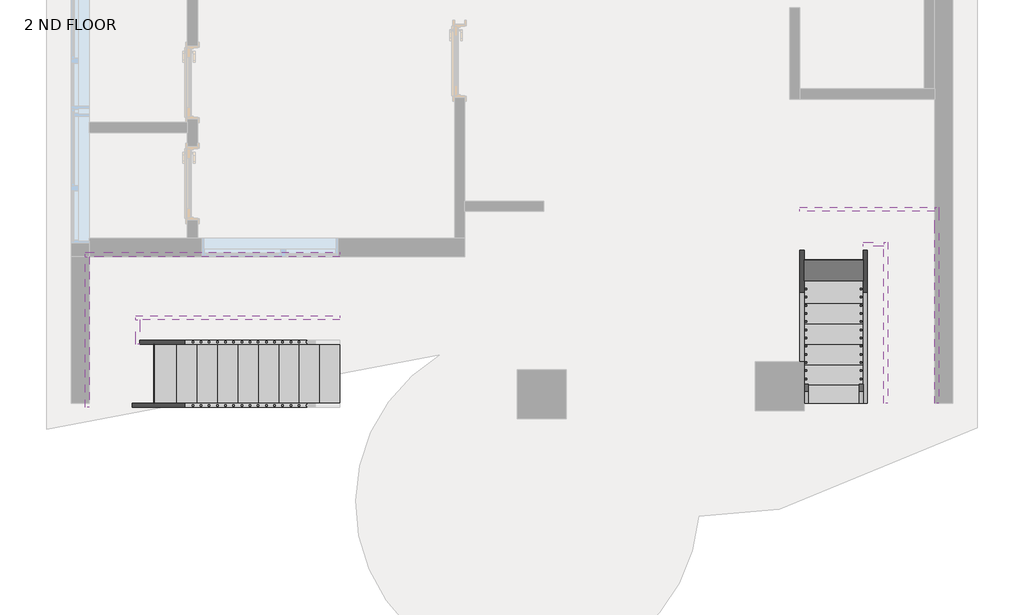
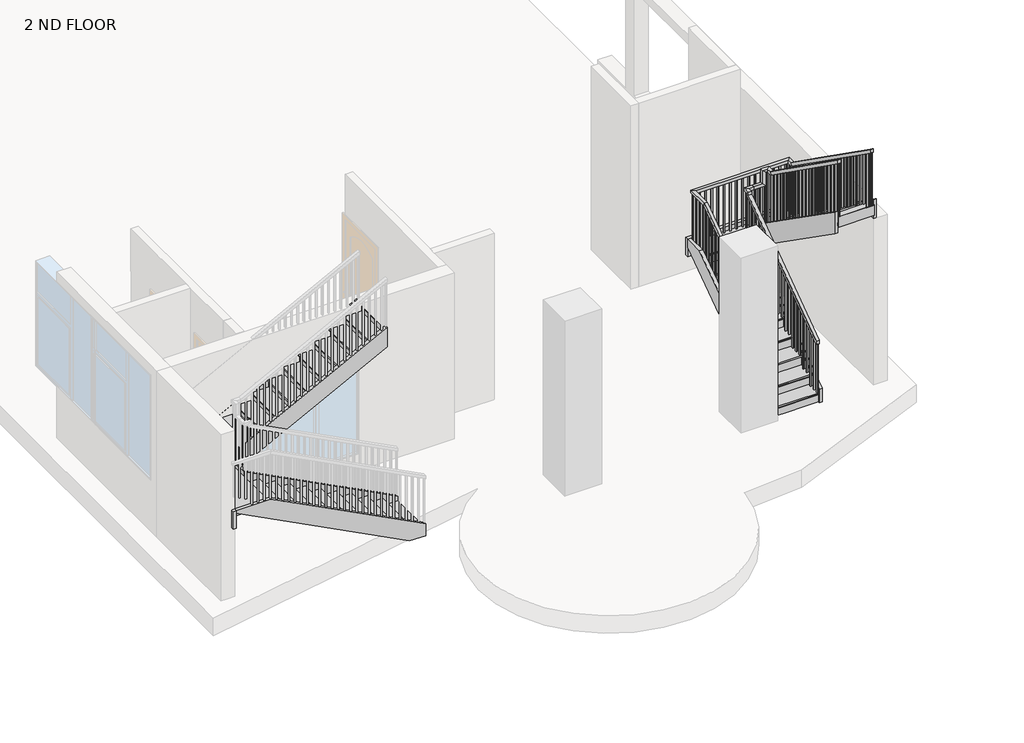
# One storey, part 4 of 4: 12 members, 2 railings, 2 stair flights.
"""IFC4 building model written with IfcOpenShell, lengths in millimetres."""

from ifc_helpers import new_model, si_unit, frame, origin, place, context, project, spatial, polyline, outline, extrude, faceted_brep, transform, mapped, element, save
from components import stair_flight_e10cbaa8, stair_flight_e23070b7

model = new_model("IFC4")

# Units and contexts
model_context = context("Model", 3, world=origin())
ifc_project = project(units=[si_unit("LENGTHUNIT", "METRE", prefix="MILLI")], contexts=[model_context])

# Site, building, storey
site = spatial("IfcSite", under=ifc_project)
building = spatial("IfcBuilding", under=site)
storey = spatial("IfcBuildingStorey", under=building, Name="2 ND FLOOR", Elevation=6400.8)

# Members
placement = place(None, origin())
element("IfcMember", 1, ObjectType="Stringer - 2\" Width", at=placement, inside=storey, context=model_context, shape_type="SweptSolid", body=[
    extrude(outline(polyline([(6400.8, -3117.2664982), (6605.3197081, -3117.2664982), (7924.8, -5663.6319738), (7924.8, -6232.5131972), (7876.2929835, -6232.5131972), (6400.8, -3385.0705974), (6400.8, -3117.2664982)])), frame((0.0, -7701.7822004, 0.0), z_axis=(0.0, 1.0, 0.0), x_axis=(0.0, 0.0, 1.0)), (0.0, 0.0, 1.0), 50.8),
])
element("IfcMember", 2, ObjectType="Stringer - 2\" Width", at=placement, inside=storey, context=model_context, shape_type="SweptSolid", body=[
    extrude(outline(polyline([(-6232.5131972, -7701.7822004), (-6283.3131972, -7701.7822004), (-6283.3131972, -5824.7082131), (-6232.5131972, -5824.7082131), (-6232.5131972, -7701.7822004)])), frame((0.0, 0.0, 7620.0), z_axis=(0.0, 0.0, 1.0), x_axis=(1.0, 0.0, 0.0)), (0.0, 0.0, 1.0), 304.8),
])
element("IfcMember", 3, ObjectType="Stringer - 2\" Width", at=placement, inside=storey, context=model_context, shape_type="SweptSolid", body=[
    extrude(outline(polyline([(7728.7136913, -6283.3131972), (7620.0, -6283.3131972), (7620.0, -5830.6202937), (9026.0106031, -3117.2664982), (9369.3015263, -3117.2664982), (7728.7136913, -6283.3131972)])), frame((0.0, -5824.7082131, 0.0), z_axis=(0.0, 1.0, 0.0), x_axis=(0.0, 0.0, 1.0)), (0.0, 0.0, 1.0), 50.8),
])
element("IfcMember", 4, ObjectType="Stringer - 2\" Width", at=placement, inside=storey, context=model_context, shape_type="SweptSolid", body=[
    extrude(outline(polyline([(6400.8, -3117.2664982), (6605.3197081, -3117.2664982), (7895.1778899, -5606.4664982), (7551.8869668, -5606.4664982), (6400.8, -3385.0705974), (6400.8, -3117.2664982)])), frame((0.0, -6914.3822004, 0.0), z_axis=(0.0, 1.0, 0.0), x_axis=(0.0, 0.0, 1.0)), (0.0, 0.0, 1.0), 50.8),
])
element("IfcMember", 5, ObjectType="Stringer - 2\" Width", at=placement, inside=storey, context=model_context, shape_type="SweptSolid", body=[
    extrude(outline(polyline([(-5606.4664982, -6914.3822004), (-5657.2664982, -6914.3822004), (-5657.2664982, -6609.5822004), (-5606.4664982, -6609.5822004), (-5606.4664982, -6914.3822004)])), frame((0.0, 0.0, 7620.0), z_axis=(0.0, 0.0, 1.0), x_axis=(1.0, 0.0, 0.0)), (0.0, 0.0, 1.0), 304.8),
])
element("IfcMember", 6, ObjectType="Stringer - 2\" Width", at=placement, inside=storey, context=model_context, shape_type="SweptSolid", body=[
    extrude(outline(polyline([(8053.1197081, -5657.2664982), (7709.8287849, -5657.2664982), (9026.0106031, -3117.2664982), (9369.3015263, -3117.2664982), (8053.1197081, -5657.2664982)])), frame((0.0, -6609.5822004, 0.0), z_axis=(0.0, 1.0, 0.0), x_axis=(0.0, 0.0, 1.0)), (0.0, 0.0, 1.0), 50.8),
])
element("IfcMember", 7, ObjectType="Stringer - 2\" Width", at=placement, inside=storey, context=model_context, shape_type="SweptSolid", body=[
    extrude(outline(polyline([(-7650.9822004, 6400.8), (-7650.9822004, 6640.099187), (-5597.981039, 8077.2), (-5263.3822004, 8077.2), (-5263.3822004, 7939.3633718), (-7461.3298744, 6400.8), (-7650.9822004, 6400.8)])), frame((2606.6891134, 0.0, 0.0), z_axis=(1.0, 0.0, 0.0), x_axis=(0.0, 1.0, 0.0)), (0.0, 0.0, 1.0), 50.8),
])
element("IfcMember", 8, ObjectType="Stringer - 2\" Width", at=placement, inside=storey, context=model_context, shape_type="SweptSolid", body=[
    extrude(outline(polyline([(2606.6891134, -5263.3822004), (2606.6891134, -5212.5822004), (4281.7311655, -5212.5822004), (4281.7311655, -5263.3822004), (2606.6891134, -5263.3822004)])), frame((0.0, 0.0, 7772.4), z_axis=(0.0, 0.0, 1.0), x_axis=(1.0, 0.0, 0.0)), (0.0, 0.0, 1.0), 304.8),
])
element("IfcMember", 9, ObjectType="Stringer - 2\" Width", at=placement, inside=storey, context=model_context, shape_type="SweptSolid", body=[
    extrude(outline(polyline([(-5212.5822004, 7920.259187), (-5212.5822004, 7772.4), (-5532.8630978, 7772.4), (-7650.9822004, 9255.0833718), (-7650.9822004, 9627.139187), (-5212.5822004, 7920.259187)])), frame((4281.7311655, 0.0, 0.0), z_axis=(1.0, 0.0, 0.0), x_axis=(0.0, 1.0, 0.0)), (0.0, 0.0, 1.0), 50.8),
])
element("IfcMember", 10, ObjectType="Stringer - 2\" Width", at=placement, inside=storey, context=model_context, shape_type="SweptSolid", body=[
    extrude(outline(polyline([(-7650.9822004, 6400.8), (-7650.9822004, 6640.099187), (-5695.1822004, 8009.159187), (-5695.1822004, 7637.1033718), (-7461.3298744, 6400.8), (-7650.9822004, 6400.8)])), frame((3394.0891134, 0.0, 0.0), z_axis=(1.0, 0.0, 0.0), x_axis=(0.0, 1.0, 0.0)), (0.0, 0.0, 1.0), 50.8),
])
element("IfcMember", 11, ObjectType="Stringer - 2\" Width", at=placement, inside=storey, context=model_context, shape_type="SweptSolid", body=[
    extrude(outline(polyline([(3394.0891134, -5695.1822004), (3394.0891134, -5644.3822004), (3648.0891134, -5644.3822004), (3648.0891134, -5695.1822004), (3394.0891134, -5695.1822004)])), frame((0.0, 0.0, 7772.4), z_axis=(0.0, 0.0, 1.0), x_axis=(1.0, 0.0, 0.0)), (0.0, 0.0, 1.0), 304.8),
])
element("IfcMember", 12, ObjectType="Stringer - 2\" Width", at=placement, inside=storey, context=model_context, shape_type="SweptSolid", body=[
    extrude(outline(polyline([(-5644.3822004, 8222.519187), (-5644.3822004, 7850.4633718), (-7650.9822004, 9255.0833718), (-7650.9822004, 9627.139187), (-5644.3822004, 8222.519187)])), frame((3648.0891134, 0.0, 0.0), z_axis=(1.0, 0.0, 0.0), x_axis=(0.0, 1.0, 0.0)), (0.0, 0.0, 1.0), 50.8),
])

# Railings
element("IfcRailing", 13, ObjectType="Handrail - Rectangular", at=placement, inside=storey, context=model_context, shape_type="SolidModel", body=[
    faceted_brep([(3343.2891134, -7650.9822004, 7493.0), (3343.2891134, -7650.9822004, 7430.7314749), (3394.0891134, -7650.9822004, 7430.7314749), (3394.0891134, -7650.9822004, 7493.0), (3343.2891134, -5720.5822004, 8861.3848101), (3343.2891134, -5669.7822004, 8835.1264116), (3394.0891134, -5669.7822004, 8835.1264116), (3394.0891134, -5720.5822004, 8861.3848101), (3343.2891134, -5720.5822004, 8915.4), (3343.2891134, -5669.7822004, 8864.6), (3394.0891134, -5669.7822004, 8864.6), (3394.0891134, -5720.5822004, 8915.4), (3343.2891134, -5593.5822004, 8915.4), (3343.2891134, -5593.5822004, 8864.6), (3394.0891134, -5644.3822004, 8864.6), (3394.0891134, -5644.3822004, 8915.4), (3470.2891134, -5593.5822004, 8915.4), (3470.2891134, -5593.5822004, 8864.6), (3470.2891134, -5644.3822004, 8864.6), (3470.2891134, -5644.3822004, 8915.4), (3622.6891134, -5593.5822004, 8915.4), (3673.4891134, -5593.5822004, 8864.6), (3673.4891134, -5644.3822004, 8864.6), (3622.6891134, -5644.3822004, 8915.4), (3622.6891134, -5593.5822004, 9147.2151899), (3673.4891134, -5593.5822004, 9096.4151899), (3673.4891134, -5644.3822004, 9096.4151899), (3622.6891134, -5644.3822004, 9147.2151899), (3749.6891134, -5593.5822004, 9147.2151899), (3749.6891134, -5593.5822004, 9096.4151899), (3698.8891134, -5644.3822004, 9096.4151899), (3698.8891134, -5644.3822004, 9147.2151899), (3749.6891134, -5720.5822004, 9147.2151899), (3749.6891134, -5736.7610126, 9096.4151899), (3698.8891134, -5736.7610126, 9096.4151899), (3698.8891134, -5720.5822004, 9147.2151899), (3749.6891134, -7650.9822004, 10515.6), (3698.8891134, -7650.9822004, 10515.6), (3698.8891134, -7650.9822004, 10453.3314749), (3749.6891134, -7650.9822004, 10453.3314749)], [[[0, 1, 2, 3]], [[1, 0, 4, 5]], [[2, 1, 5, 6]], [[3, 2, 6, 7]], [[0, 3, 7, 4]], [[5, 4, 8, 9]], [[6, 5, 9, 10]], [[7, 6, 10, 11]], [[4, 7, 11, 8]], [[9, 8, 12, 13]], [[10, 9, 13, 14]], [[11, 10, 14, 15]], [[8, 11, 15, 12]], [[13, 12, 16, 17]], [[14, 13, 17, 18]], [[15, 14, 18, 19]], [[12, 15, 19, 16]], [[17, 16, 20, 21]], [[18, 17, 21, 22]], [[19, 18, 22, 23]], [[16, 19, 23, 20]], [[21, 20, 24, 25]], [[22, 21, 25, 26]], [[23, 22, 26, 27]], [[20, 23, 27, 24]], [[25, 24, 28, 29]], [[26, 25, 29, 30]], [[27, 26, 30, 31]], [[24, 27, 31, 28]], [[29, 28, 32, 33]], [[30, 29, 33, 34]], [[31, 30, 34, 35]], [[28, 31, 35, 32]], [[36, 37, 38, 39]], [[33, 32, 36, 39]], [[34, 33, 39, 38]], [[35, 34, 38, 37]], [[32, 35, 37, 36]]]),
    extrude(outline(polyline([(-7558.9072004, 10388.0631205), (-7539.8572004, 10374.559323), (-7539.8572004, 9423.4), (-7558.9072004, 9423.4), (-7558.9072004, 10388.0631205)])), frame((3714.7641134, 0.0, 0.0), z_axis=(1.0, 0.0, 0.0), x_axis=(0.0, 1.0, 0.0)), (0.0, 0.0, 1.0), 19.05),
    extrude(outline(polyline([(-7457.3072004, 10316.0428673), (-7438.2572004, 10302.5390699), (-7438.2572004, 9423.4), (-7457.3072004, 9423.4), (-7457.3072004, 10316.0428673)])), frame((3714.7641134, 0.0, 0.0), z_axis=(1.0, 0.0, 0.0), x_axis=(0.0, 1.0, 0.0)), (0.0, 0.0, 1.0), 19.05),
    extrude(outline(polyline([(-7355.7072004, 10244.0226142), (-7336.6572004, 10230.5188167), (-7336.6572004, 9245.6), (-7355.7072004, 9245.6), (-7355.7072004, 10244.0226142)])), frame((3714.7641134, 0.0, 0.0), z_axis=(1.0, 0.0, 0.0), x_axis=(0.0, 1.0, 0.0)), (0.0, 0.0, 1.0), 19.05),
    extrude(outline(polyline([(-7254.1072004, 10172.002361), (-7235.0572004, 10158.4985635), (-7235.0572004, 9245.6), (-7254.1072004, 9245.6), (-7254.1072004, 10172.002361)])), frame((3714.7641134, 0.0, 0.0), z_axis=(1.0, 0.0, 0.0), x_axis=(0.0, 1.0, 0.0)), (0.0, 0.0, 1.0), 19.05),
    extrude(outline(polyline([(-7152.5072004, 10099.9821078), (-7133.4572004, 10086.4783104), (-7133.4572004, 9067.8), (-7152.5072004, 9067.8), (-7152.5072004, 10099.9821078)])), frame((3714.7641134, 0.0, 0.0), z_axis=(1.0, 0.0, 0.0), x_axis=(0.0, 1.0, 0.0)), (0.0, 0.0, 1.0), 19.05),
    extrude(outline(polyline([(-7050.9072004, 10027.9618547), (-7031.8572004, 10014.4580572), (-7031.8572004, 9067.8), (-7050.9072004, 9067.8), (-7050.9072004, 10027.9618547)])), frame((3714.7641134, 0.0, 0.0), z_axis=(1.0, 0.0, 0.0), x_axis=(0.0, 1.0, 0.0)), (0.0, 0.0, 1.0), 19.05),
    extrude(outline(polyline([(-6949.3072004, 9955.9416015), (-6930.2572004, 9942.437804), (-6930.2572004, 9067.8), (-6949.3072004, 9067.8), (-6949.3072004, 9955.9416015)])), frame((3714.7641134, 0.0, 0.0), z_axis=(1.0, 0.0, 0.0), x_axis=(0.0, 1.0, 0.0)), (0.0, 0.0, 1.0), 19.05),
    extrude(outline(polyline([(-6847.7072004, 9883.9213483), (-6828.6572004, 9870.4175509), (-6828.6572004, 8890.0), (-6847.7072004, 8890.0), (-6847.7072004, 9883.9213483)])), frame((3714.7641134, 0.0, 0.0), z_axis=(1.0, 0.0, 0.0), x_axis=(0.0, 1.0, 0.0)), (0.0, 0.0, 1.0), 19.05),
    extrude(outline(polyline([(-6746.1072004, 9811.9010952), (-6727.0572004, 9798.3972977), (-6727.0572004, 8890.0), (-6746.1072004, 8890.0), (-6746.1072004, 9811.9010952)])), frame((3714.7641134, 0.0, 0.0), z_axis=(1.0, 0.0, 0.0), x_axis=(0.0, 1.0, 0.0)), (0.0, 0.0, 1.0), 19.05),
    extrude(outline(polyline([(-6644.5072004, 9739.880842), (-6625.4572004, 9726.3770445), (-6625.4572004, 8712.2), (-6644.5072004, 8712.2), (-6644.5072004, 9739.880842)])), frame((3714.7641134, 0.0, 0.0), z_axis=(1.0, 0.0, 0.0), x_axis=(0.0, 1.0, 0.0)), (0.0, 0.0, 1.0), 19.05),
    extrude(outline(polyline([(-6542.9072004, 9667.8605888), (-6523.8572004, 9654.3567914), (-6523.8572004, 8712.2), (-6542.9072004, 8712.2), (-6542.9072004, 9667.8605888)])), frame((3714.7641134, 0.0, 0.0), z_axis=(1.0, 0.0, 0.0), x_axis=(0.0, 1.0, 0.0)), (0.0, 0.0, 1.0), 19.05),
    extrude(outline(polyline([(-6441.3072004, 9595.8403357), (-6422.2572004, 9582.3365382), (-6422.2572004, 8712.2), (-6441.3072004, 8712.2), (-6441.3072004, 9595.8403357)])), frame((3714.7641134, 0.0, 0.0), z_axis=(1.0, 0.0, 0.0), x_axis=(0.0, 1.0, 0.0)), (0.0, 0.0, 1.0), 19.05),
    extrude(outline(polyline([(-6339.7072004, 9523.8200825), (-6320.6572004, 9510.316285), (-6320.6572004, 8534.4), (-6339.7072004, 8534.4), (-6339.7072004, 9523.8200825)])), frame((3714.7641134, 0.0, 0.0), z_axis=(1.0, 0.0, 0.0), x_axis=(0.0, 1.0, 0.0)), (0.0, 0.0, 1.0), 19.05),
    extrude(outline(polyline([(-6238.1072004, 9451.7998293), (-6219.0572004, 9438.2960319), (-6219.0572004, 8534.4), (-6238.1072004, 8534.4), (-6238.1072004, 9451.7998293)])), frame((3714.7641134, 0.0, 0.0), z_axis=(1.0, 0.0, 0.0), x_axis=(0.0, 1.0, 0.0)), (0.0, 0.0, 1.0), 19.05),
    extrude(outline(polyline([(-6136.5072004, 9379.7795762), (-6117.4572004, 9366.2757787), (-6117.4572004, 8356.6), (-6136.5072004, 8356.6), (-6136.5072004, 9379.7795762)])), frame((3714.7641134, 0.0, 0.0), z_axis=(1.0, 0.0, 0.0), x_axis=(0.0, 1.0, 0.0)), (0.0, 0.0, 1.0), 19.05),
    extrude(outline(polyline([(-6034.9072004, 9307.759323), (-6015.8572004, 9294.2555255), (-6015.8572004, 8356.6), (-6034.9072004, 8356.6), (-6034.9072004, 9307.759323)])), frame((3714.7641134, 0.0, 0.0), z_axis=(1.0, 0.0, 0.0), x_axis=(0.0, 1.0, 0.0)), (0.0, 0.0, 1.0), 19.05),
    extrude(outline(polyline([(-5933.3072004, 9235.7390699), (-5914.2572004, 9222.2352724), (-5914.2572004, 8356.6), (-5933.3072004, 8356.6), (-5933.3072004, 9235.7390699)])), frame((3714.7641134, 0.0, 0.0), z_axis=(1.0, 0.0, 0.0), x_axis=(0.0, 1.0, 0.0)), (0.0, 0.0, 1.0), 19.05),
    extrude(outline(polyline([(-5831.7072004, 9163.7188167), (-5812.6572004, 9150.2150192), (-5812.6572004, 8178.8), (-5831.7072004, 8178.8), (-5831.7072004, 9163.7188167)])), frame((3714.7641134, 0.0, 0.0), z_axis=(1.0, 0.0, 0.0), x_axis=(0.0, 1.0, 0.0)), (0.0, 0.0, 1.0), 19.05),
    extrude(outline(polyline([(-5730.1072004, 9091.6985635), (-5711.0572004, 9078.1947661), (-5711.0572004, 8178.8), (-5730.1072004, 8178.8), (-5730.1072004, 9091.6985635)])), frame((3714.7641134, 0.0, 0.0), z_axis=(1.0, 0.0, 0.0), x_axis=(0.0, 1.0, 0.0)), (0.0, 0.0, 1.0), 19.05),
    extrude(outline(polyline([(3663.9641134, -5628.5072004), (3663.9641134, -5609.4572004), (3683.0141134, -5609.4572004), (3683.0141134, -5628.5072004), (3663.9641134, -5628.5072004)])), frame((0.0, 0.0, 8001.0), z_axis=(0.0, 0.0, 1.0), x_axis=(1.0, 0.0, 0.0)), (0.0, 0.0, 1.0), 1095.4151899),
    extrude(outline(polyline([(3562.3641134, -5628.5072004), (3562.3641134, -5609.4572004), (3581.4141134, -5609.4572004), (3581.4141134, -5628.5072004), (3562.3641134, -5628.5072004)])), frame((0.0, 0.0, 8001.0), z_axis=(0.0, 0.0, 1.0), x_axis=(1.0, 0.0, 0.0)), (0.0, 0.0, 1.0), 863.6),
    extrude(outline(polyline([(3460.7641134, -5628.5072004), (3460.7641134, -5609.4572004), (3479.8141134, -5609.4572004), (3479.8141134, -5628.5072004), (3460.7641134, -5628.5072004)])), frame((0.0, 0.0, 8001.0), z_axis=(0.0, 0.0, 1.0), x_axis=(1.0, 0.0, 0.0)), (0.0, 0.0, 1.0), 863.6),
    extrude(outline(polyline([(-5730.1072004, 8792.3643863), (-5711.0572004, 8805.8681838), (-5711.0572004, 7823.2), (-5730.1072004, 7823.2), (-5730.1072004, 8792.3643863)])), frame((3359.1641134, 0.0, 0.0), z_axis=(1.0, 0.0, 0.0), x_axis=(0.0, 1.0, 0.0)), (0.0, 0.0, 1.0), 19.05),
    extrude(outline(polyline([(-5831.7072004, 8720.3441331), (-5812.6572004, 8733.8479306), (-5812.6572004, 7823.2), (-5831.7072004, 7823.2), (-5831.7072004, 8720.3441331)])), frame((3359.1641134, 0.0, 0.0), z_axis=(1.0, 0.0, 0.0), x_axis=(0.0, 1.0, 0.0)), (0.0, 0.0, 1.0), 19.05),
    extrude(outline(polyline([(-5933.3072004, 8648.32388), (-5914.2572004, 8661.8276774), (-5914.2572004, 7645.4), (-5933.3072004, 7645.4), (-5933.3072004, 8648.32388)])), frame((3359.1641134, 0.0, 0.0), z_axis=(1.0, 0.0, 0.0), x_axis=(0.0, 1.0, 0.0)), (0.0, 0.0, 1.0), 19.05),
    extrude(outline(polyline([(-6034.9072004, 8576.3036268), (-6015.8572004, 8589.8074243), (-6015.8572004, 7645.4), (-6034.9072004, 7645.4), (-6034.9072004, 8576.3036268)])), frame((3359.1641134, 0.0, 0.0), z_axis=(1.0, 0.0, 0.0), x_axis=(0.0, 1.0, 0.0)), (0.0, 0.0, 1.0), 19.05),
    extrude(outline(polyline([(-6136.5072004, 8504.2833736), (-6117.4572004, 8517.7871711), (-6117.4572004, 7645.4), (-6136.5072004, 7645.4), (-6136.5072004, 8504.2833736)])), frame((3359.1641134, 0.0, 0.0), z_axis=(1.0, 0.0, 0.0), x_axis=(0.0, 1.0, 0.0)), (0.0, 0.0, 1.0), 19.05),
    extrude(outline(polyline([(-6238.1072004, 8432.2631205), (-6219.0572004, 8445.766918), (-6219.0572004, 7467.6), (-6238.1072004, 7467.6), (-6238.1072004, 8432.2631205)])), frame((3359.1641134, 0.0, 0.0), z_axis=(1.0, 0.0, 0.0), x_axis=(0.0, 1.0, 0.0)), (0.0, 0.0, 1.0), 19.05),
    extrude(outline(polyline([(-6339.7072004, 8360.2428673), (-6320.6572004, 8373.7466648), (-6320.6572004, 7467.6), (-6339.7072004, 7467.6), (-6339.7072004, 8360.2428673)])), frame((3359.1641134, 0.0, 0.0), z_axis=(1.0, 0.0, 0.0), x_axis=(0.0, 1.0, 0.0)), (0.0, 0.0, 1.0), 19.05),
    extrude(outline(polyline([(-6441.3072004, 8288.2226142), (-6422.2572004, 8301.7264116), (-6422.2572004, 7289.8), (-6441.3072004, 7289.8), (-6441.3072004, 8288.2226142)])), frame((3359.1641134, 0.0, 0.0), z_axis=(1.0, 0.0, 0.0), x_axis=(0.0, 1.0, 0.0)), (0.0, 0.0, 1.0), 19.05),
    extrude(outline(polyline([(-6542.9072004, 8216.202361), (-6523.8572004, 8229.7061585), (-6523.8572004, 7289.8), (-6542.9072004, 7289.8), (-6542.9072004, 8216.202361)])), frame((3359.1641134, 0.0, 0.0), z_axis=(1.0, 0.0, 0.0), x_axis=(0.0, 1.0, 0.0)), (0.0, 0.0, 1.0), 19.05),
    extrude(outline(polyline([(-6644.5072004, 8144.1821078), (-6625.4572004, 8157.6859053), (-6625.4572004, 7289.8), (-6644.5072004, 7289.8), (-6644.5072004, 8144.1821078)])), frame((3359.1641134, 0.0, 0.0), z_axis=(1.0, 0.0, 0.0), x_axis=(0.0, 1.0, 0.0)), (0.0, 0.0, 1.0), 19.05),
    extrude(outline(polyline([(-6746.1072004, 8072.1618547), (-6727.0572004, 8085.6656521), (-6727.0572004, 7112.0), (-6746.1072004, 7112.0), (-6746.1072004, 8072.1618547)])), frame((3359.1641134, 0.0, 0.0), z_axis=(1.0, 0.0, 0.0), x_axis=(0.0, 1.0, 0.0)), (0.0, 0.0, 1.0), 19.05),
    extrude(outline(polyline([(-6847.7072004, 8000.1416015), (-6828.6572004, 8013.645399), (-6828.6572004, 7112.0), (-6847.7072004, 7112.0), (-6847.7072004, 8000.1416015)])), frame((3359.1641134, 0.0, 0.0), z_axis=(1.0, 0.0, 0.0), x_axis=(0.0, 1.0, 0.0)), (0.0, 0.0, 1.0), 19.05),
    extrude(outline(polyline([(-6949.3072004, 7928.1213483), (-6930.2572004, 7941.6251458), (-6930.2572004, 6934.2), (-6949.3072004, 6934.2), (-6949.3072004, 7928.1213483)])), frame((3359.1641134, 0.0, 0.0), z_axis=(1.0, 0.0, 0.0), x_axis=(0.0, 1.0, 0.0)), (0.0, 0.0, 1.0), 19.05),
    extrude(outline(polyline([(-7050.9072004, 7856.1010952), (-7031.8572004, 7869.6048926), (-7031.8572004, 6934.2), (-7050.9072004, 6934.2), (-7050.9072004, 7856.1010952)])), frame((3359.1641134, 0.0, 0.0), z_axis=(1.0, 0.0, 0.0), x_axis=(0.0, 1.0, 0.0)), (0.0, 0.0, 1.0), 19.05),
    extrude(outline(polyline([(-7152.5072004, 7784.080842), (-7133.4572004, 7797.5846395), (-7133.4572004, 6934.2), (-7152.5072004, 6934.2), (-7152.5072004, 7784.080842)])), frame((3359.1641134, 0.0, 0.0), z_axis=(1.0, 0.0, 0.0), x_axis=(0.0, 1.0, 0.0)), (0.0, 0.0, 1.0), 19.05),
    extrude(outline(polyline([(-7254.1072004, 7712.0605888), (-7235.0572004, 7725.5643863), (-7235.0572004, 6756.4), (-7254.1072004, 6756.4), (-7254.1072004, 7712.0605888)])), frame((3359.1641134, 0.0, 0.0), z_axis=(1.0, 0.0, 0.0), x_axis=(0.0, 1.0, 0.0)), (0.0, 0.0, 1.0), 19.05),
    extrude(outline(polyline([(-7355.7072004, 7640.0403357), (-7336.6572004, 7653.5441331), (-7336.6572004, 6756.4), (-7355.7072004, 6756.4), (-7355.7072004, 7640.0403357)])), frame((3359.1641134, 0.0, 0.0), z_axis=(1.0, 0.0, 0.0), x_axis=(0.0, 1.0, 0.0)), (0.0, 0.0, 1.0), 19.05),
    extrude(outline(polyline([(-7457.3072004, 7568.0200825), (-7438.2572004, 7581.52388), (-7438.2572004, 6578.6), (-7457.3072004, 6578.6), (-7457.3072004, 7568.0200825)])), frame((3359.1641134, 0.0, 0.0), z_axis=(1.0, 0.0, 0.0), x_axis=(0.0, 1.0, 0.0)), (0.0, 0.0, 1.0), 19.05),
    extrude(outline(polyline([(-7558.9072004, 7495.9998293), (-7539.8572004, 7509.5036268), (-7539.8572004, 6578.6), (-7558.9072004, 6578.6), (-7558.9072004, 7495.9998293)])), frame((3359.1641134, 0.0, 0.0), z_axis=(1.0, 0.0, 0.0), x_axis=(0.0, 1.0, 0.0)), (0.0, 0.0, 1.0), 19.05),
    extrude(outline(polyline([(3714.7641134, -5628.5072004), (3714.7641134, -5609.4572004), (3733.8141134, -5609.4572004), (3733.8141134, -5628.5072004), (3714.7641134, -5628.5072004)])), frame((0.0, 0.0, 8001.0), z_axis=(0.0, 0.0, 1.0), x_axis=(1.0, 0.0, 0.0)), (0.0, 0.0, 1.0), 1095.4151899),
    extrude(outline(polyline([(3378.2141134, -5628.5072004), (3359.1641134, -5628.5072004), (3359.1641134, -5609.4572004), (3378.2141134, -5609.4572004), (3378.2141134, -5628.5072004)])), frame((0.0, 0.0, 8001.0), z_axis=(0.0, 0.0, 1.0), x_axis=(1.0, 0.0, 0.0)), (0.0, 0.0, 1.0), 863.6),
    extrude(outline(polyline([(-7650.9822004, 10453.3314749), (-7631.9322004, 10439.8276774), (-7631.9322004, 9423.4), (-7650.9822004, 9423.4), (-7650.9822004, 10453.3314749)])), frame((3714.7641134, 0.0, 0.0), z_axis=(1.0, 0.0, 0.0), x_axis=(0.0, 1.0, 0.0)), (0.0, 0.0, 1.0), 19.05),
    extrude(outline(polyline([(-7650.9822004, 7430.7314749), (-7631.9322004, 7444.2352724), (-7631.9322004, 6578.6), (-7650.9822004, 6578.6), (-7650.9822004, 7430.7314749)])), frame((3359.1641134, 0.0, 0.0), z_axis=(1.0, 0.0, 0.0), x_axis=(0.0, 1.0, 0.0)), (0.0, 0.0, 1.0), 19.05),
])
element("IfcRailing", 14, ObjectType="Handrail - Rectangular", at=placement, inside=storey, context=model_context, shape_type="SolidModel", body=[
    faceted_brep([(2657.4891134, -7650.9822004, 7493.0), (2657.4891134, -7650.9822004, 7430.7314749), (2708.2891134, -7650.9822004, 7430.7314749), (2708.2891134, -7650.9822004, 7493.0), (2657.4891134, -5644.3822004, 8915.4), (2657.4891134, -5628.2033882, 8864.6), (2708.2891134, -5628.2033882, 8864.6), (2708.2891134, -5644.3822004, 8915.4), (2657.4891134, -5263.3822004, 8915.4), (2657.4891134, -5263.3822004, 8864.6), (2708.2891134, -5314.1822004, 8864.6), (2708.2891134, -5314.1822004, 8915.4), (4281.7311655, -5263.3822004, 8915.4), (4281.7311655, -5263.3822004, 8864.6), (4230.9311655, -5314.1822004, 8864.6), (4230.9311655, -5314.1822004, 8915.4), (4281.7311655, -5393.5572004, 8915.4), (4281.7311655, -5409.7360126, 8864.6), (4230.9311655, -5409.7360126, 8864.6), (4230.9311655, -5393.5572004, 8915.4), (4281.7311655, -7650.9822004, 10515.6), (4230.9311655, -7650.9822004, 10515.6), (4230.9311655, -7650.9822004, 10453.3314749), (4281.7311655, -7650.9822004, 10453.3314749)], [[[0, 1, 2, 3]], [[1, 0, 4, 5]], [[2, 1, 5, 6]], [[3, 2, 6, 7]], [[0, 3, 7, 4]], [[5, 4, 8, 9]], [[6, 5, 9, 10]], [[7, 6, 10, 11]], [[4, 7, 11, 8]], [[9, 8, 12, 13]], [[10, 9, 13, 14]], [[11, 10, 14, 15]], [[8, 11, 15, 12]], [[13, 12, 16, 17]], [[14, 13, 17, 18]], [[15, 14, 18, 19]], [[12, 15, 19, 16]], [[20, 21, 22, 23]], [[17, 16, 20, 23]], [[18, 17, 23, 22]], [[19, 18, 22, 21]], [[16, 19, 21, 20]]]),
    extrude(outline(polyline([(-7616.0572004, 10428.5745129), (-7616.0572004, 9423.4), (-7635.1072004, 9423.4), (-7635.1072004, 10442.0783104), (-7616.0572004, 10428.5745129)])), frame((4246.8061655, 0.0, 0.0), z_axis=(1.0, 0.0, 0.0), x_axis=(0.0, 1.0, 0.0)), (0.0, 0.0, 1.0), 19.05),
    extrude(outline(polyline([(-7514.4572004, 10356.5542597), (-7514.4572004, 9423.4), (-7533.5072004, 9423.4), (-7533.5072004, 10370.0580572), (-7514.4572004, 10356.5542597)])), frame((4246.8061655, 0.0, 0.0), z_axis=(1.0, 0.0, 0.0), x_axis=(0.0, 1.0, 0.0)), (0.0, 0.0, 1.0), 19.05),
    extrude(outline(polyline([(-7412.8572004, 10284.5340066), (-7412.8572004, 9423.4), (-7431.9072004, 9423.4), (-7431.9072004, 10298.037804), (-7412.8572004, 10284.5340066)])), frame((4246.8061655, 0.0, 0.0), z_axis=(1.0, 0.0, 0.0), x_axis=(0.0, 1.0, 0.0)), (0.0, 0.0, 1.0), 19.05),
    extrude(outline(polyline([(-7311.2572004, 10212.5137534), (-7311.2572004, 9245.6), (-7330.3072004, 9245.6), (-7330.3072004, 10226.0175509), (-7311.2572004, 10212.5137534)])), frame((4246.8061655, 0.0, 0.0), z_axis=(1.0, 0.0, 0.0), x_axis=(0.0, 1.0, 0.0)), (0.0, 0.0, 1.0), 19.05),
    extrude(outline(polyline([(-7209.6572004, 10140.4935002), (-7209.6572004, 9245.6), (-7228.7072004, 9245.6), (-7228.7072004, 10153.9972977), (-7209.6572004, 10140.4935002)])), frame((4246.8061655, 0.0, 0.0), z_axis=(1.0, 0.0, 0.0), x_axis=(0.0, 1.0, 0.0)), (0.0, 0.0, 1.0), 19.05),
    extrude(outline(polyline([(-7108.0572004, 10068.4732471), (-7108.0572004, 9067.8), (-7127.1072004, 9067.8), (-7127.1072004, 10081.9770445), (-7108.0572004, 10068.4732471)])), frame((4246.8061655, 0.0, 0.0), z_axis=(1.0, 0.0, 0.0), x_axis=(0.0, 1.0, 0.0)), (0.0, 0.0, 1.0), 19.05),
    extrude(outline(polyline([(-7006.4572004, 9996.4529939), (-7006.4572004, 9067.8), (-7025.5072004, 9067.8), (-7025.5072004, 10009.9567914), (-7006.4572004, 9996.4529939)])), frame((4246.8061655, 0.0, 0.0), z_axis=(1.0, 0.0, 0.0), x_axis=(0.0, 1.0, 0.0)), (0.0, 0.0, 1.0), 19.05),
    extrude(outline(polyline([(-6904.8572004, 9924.4327407), (-6904.8572004, 9067.8), (-6923.9072004, 9067.8), (-6923.9072004, 9937.9365382), (-6904.8572004, 9924.4327407)])), frame((4246.8061655, 0.0, 0.0), z_axis=(1.0, 0.0, 0.0), x_axis=(0.0, 1.0, 0.0)), (0.0, 0.0, 1.0), 19.05),
    extrude(outline(polyline([(-6803.2572004, 9852.4124876), (-6803.2572004, 8890.0), (-6822.3072004, 8890.0), (-6822.3072004, 9865.916285), (-6803.2572004, 9852.4124876)])), frame((4246.8061655, 0.0, 0.0), z_axis=(1.0, 0.0, 0.0), x_axis=(0.0, 1.0, 0.0)), (0.0, 0.0, 1.0), 19.05),
    extrude(outline(polyline([(-6701.6572004, 9780.3922344), (-6701.6572004, 8890.0), (-6720.7072004, 8890.0), (-6720.7072004, 9793.8960319), (-6701.6572004, 9780.3922344)])), frame((4246.8061655, 0.0, 0.0), z_axis=(1.0, 0.0, 0.0), x_axis=(0.0, 1.0, 0.0)), (0.0, 0.0, 1.0), 19.05),
    extrude(outline(polyline([(-6600.0572004, 9708.3719812), (-6600.0572004, 8712.2), (-6619.1072004, 8712.2), (-6619.1072004, 9721.8757787), (-6600.0572004, 9708.3719812)])), frame((4246.8061655, 0.0, 0.0), z_axis=(1.0, 0.0, 0.0), x_axis=(0.0, 1.0, 0.0)), (0.0, 0.0, 1.0), 19.05),
    extrude(outline(polyline([(-6498.4572004, 9636.3517281), (-6498.4572004, 8712.2), (-6517.5072004, 8712.2), (-6517.5072004, 9649.8555255), (-6498.4572004, 9636.3517281)])), frame((4246.8061655, 0.0, 0.0), z_axis=(1.0, 0.0, 0.0), x_axis=(0.0, 1.0, 0.0)), (0.0, 0.0, 1.0), 19.05),
    extrude(outline(polyline([(-6396.8572004, 9564.3314749), (-6396.8572004, 8712.2), (-6415.9072004, 8712.2), (-6415.9072004, 9577.8352724), (-6396.8572004, 9564.3314749)])), frame((4246.8061655, 0.0, 0.0), z_axis=(1.0, 0.0, 0.0), x_axis=(0.0, 1.0, 0.0)), (0.0, 0.0, 1.0), 19.05),
    extrude(outline(polyline([(-6295.2572004, 9492.3112217), (-6295.2572004, 8534.4), (-6314.3072004, 8534.4), (-6314.3072004, 9505.8150192), (-6295.2572004, 9492.3112217)])), frame((4246.8061655, 0.0, 0.0), z_axis=(1.0, 0.0, 0.0), x_axis=(0.0, 1.0, 0.0)), (0.0, 0.0, 1.0), 19.05),
    extrude(outline(polyline([(-6193.6572004, 9420.2909686), (-6193.6572004, 8534.4), (-6212.7072004, 8534.4), (-6212.7072004, 9433.7947661), (-6193.6572004, 9420.2909686)])), frame((4246.8061655, 0.0, 0.0), z_axis=(1.0, 0.0, 0.0), x_axis=(0.0, 1.0, 0.0)), (0.0, 0.0, 1.0), 19.05),
    extrude(outline(polyline([(-6092.0572004, 9348.2707154), (-6092.0572004, 8356.6), (-6111.1072004, 8356.6), (-6111.1072004, 9361.7745129), (-6092.0572004, 9348.2707154)])), frame((4246.8061655, 0.0, 0.0), z_axis=(1.0, 0.0, 0.0), x_axis=(0.0, 1.0, 0.0)), (0.0, 0.0, 1.0), 19.05),
    extrude(outline(polyline([(-5990.4572004, 9276.2504623), (-5990.4572004, 8356.6), (-6009.5072004, 8356.6), (-6009.5072004, 9289.7542597), (-5990.4572004, 9276.2504623)])), frame((4246.8061655, 0.0, 0.0), z_axis=(1.0, 0.0, 0.0), x_axis=(0.0, 1.0, 0.0)), (0.0, 0.0, 1.0), 19.05),
    extrude(outline(polyline([(-5888.8572004, 9204.2302091), (-5888.8572004, 8356.6), (-5907.9072004, 8356.6), (-5907.9072004, 9217.7340066), (-5888.8572004, 9204.2302091)])), frame((4246.8061655, 0.0, 0.0), z_axis=(1.0, 0.0, 0.0), x_axis=(0.0, 1.0, 0.0)), (0.0, 0.0, 1.0), 19.05),
    extrude(outline(polyline([(-5787.2572004, 9132.2099559), (-5787.2572004, 8178.8), (-5806.3072004, 8178.8), (-5806.3072004, 9145.7137534), (-5787.2572004, 9132.2099559)])), frame((4246.8061655, 0.0, 0.0), z_axis=(1.0, 0.0, 0.0), x_axis=(0.0, 1.0, 0.0)), (0.0, 0.0, 1.0), 19.05),
    extrude(outline(polyline([(-5685.6572004, 9060.1897028), (-5685.6572004, 8178.8), (-5704.7072004, 8178.8), (-5704.7072004, 9073.6935002), (-5685.6572004, 9060.1897028)])), frame((4246.8061655, 0.0, 0.0), z_axis=(1.0, 0.0, 0.0), x_axis=(0.0, 1.0, 0.0)), (0.0, 0.0, 1.0), 19.05),
    extrude(outline(polyline([(-5584.0572004, 8988.1694496), (-5584.0572004, 8001.0), (-5603.1072004, 8001.0), (-5603.1072004, 9001.6732471), (-5584.0572004, 8988.1694496)])), frame((4246.8061655, 0.0, 0.0), z_axis=(1.0, 0.0, 0.0), x_axis=(0.0, 1.0, 0.0)), (0.0, 0.0, 1.0), 19.05),
    extrude(outline(polyline([(-5482.4572004, 8916.1491964), (-5482.4572004, 8001.0), (-5501.5072004, 8001.0), (-5501.5072004, 8929.6529939), (-5482.4572004, 8916.1491964)])), frame((4246.8061655, 0.0, 0.0), z_axis=(1.0, 0.0, 0.0), x_axis=(0.0, 1.0, 0.0)), (0.0, 0.0, 1.0), 19.05),
    extrude(outline(polyline([(4265.8561655, -5380.8572004), (4265.8561655, -5399.9072004), (4246.8061655, -5399.9072004), (4246.8061655, -5380.8572004), (4265.8561655, -5380.8572004)])), frame((0.0, 0.0, 8001.0), z_axis=(0.0, 0.0, 1.0), x_axis=(1.0, 0.0, 0.0)), (0.0, 0.0, 1.0), 863.6),
    extrude(outline(polyline([(4197.3641134, -5279.2572004), (4216.4141134, -5279.2572004), (4216.4141134, -5298.3072004), (4197.3641134, -5298.3072004), (4197.3641134, -5279.2572004)])), frame((0.0, 0.0, 8001.0), z_axis=(0.0, 0.0, 1.0), x_axis=(1.0, 0.0, 0.0)), (0.0, 0.0, 1.0), 863.6),
    extrude(outline(polyline([(4095.7641134, -5279.2572004), (4114.8141134, -5279.2572004), (4114.8141134, -5298.3072004), (4095.7641134, -5298.3072004), (4095.7641134, -5279.2572004)])), frame((0.0, 0.0, 8001.0), z_axis=(0.0, 0.0, 1.0), x_axis=(1.0, 0.0, 0.0)), (0.0, 0.0, 1.0), 863.6),
    extrude(outline(polyline([(3994.1641134, -5279.2572004), (4013.2141134, -5279.2572004), (4013.2141134, -5298.3072004), (3994.1641134, -5298.3072004), (3994.1641134, -5279.2572004)])), frame((0.0, 0.0, 8001.0), z_axis=(0.0, 0.0, 1.0), x_axis=(1.0, 0.0, 0.0)), (0.0, 0.0, 1.0), 863.6),
    extrude(outline(polyline([(3892.5641134, -5279.2572004), (3911.6141134, -5279.2572004), (3911.6141134, -5298.3072004), (3892.5641134, -5298.3072004), (3892.5641134, -5279.2572004)])), frame((0.0, 0.0, 8001.0), z_axis=(0.0, 0.0, 1.0), x_axis=(1.0, 0.0, 0.0)), (0.0, 0.0, 1.0), 863.6),
    extrude(outline(polyline([(3790.9641134, -5279.2572004), (3810.0141134, -5279.2572004), (3810.0141134, -5298.3072004), (3790.9641134, -5298.3072004), (3790.9641134, -5279.2572004)])), frame((0.0, 0.0, 8001.0), z_axis=(0.0, 0.0, 1.0), x_axis=(1.0, 0.0, 0.0)), (0.0, 0.0, 1.0), 863.6),
    extrude(outline(polyline([(3689.3641134, -5279.2572004), (3708.4141134, -5279.2572004), (3708.4141134, -5298.3072004), (3689.3641134, -5298.3072004), (3689.3641134, -5279.2572004)])), frame((0.0, 0.0, 8001.0), z_axis=(0.0, 0.0, 1.0), x_axis=(1.0, 0.0, 0.0)), (0.0, 0.0, 1.0), 863.6),
    extrude(outline(polyline([(3587.7641134, -5279.2572004), (3606.8141134, -5279.2572004), (3606.8141134, -5298.3072004), (3587.7641134, -5298.3072004), (3587.7641134, -5279.2572004)])), frame((0.0, 0.0, 8001.0), z_axis=(0.0, 0.0, 1.0), x_axis=(1.0, 0.0, 0.0)), (0.0, 0.0, 1.0), 863.6),
    extrude(outline(polyline([(3486.1641134, -5279.2572004), (3505.2141134, -5279.2572004), (3505.2141134, -5298.3072004), (3486.1641134, -5298.3072004), (3486.1641134, -5279.2572004)])), frame((0.0, 0.0, 8001.0), z_axis=(0.0, 0.0, 1.0), x_axis=(1.0, 0.0, 0.0)), (0.0, 0.0, 1.0), 863.6),
    extrude(outline(polyline([(3384.5641134, -5279.2572004), (3403.6141134, -5279.2572004), (3403.6141134, -5298.3072004), (3384.5641134, -5298.3072004), (3384.5641134, -5279.2572004)])), frame((0.0, 0.0, 8001.0), z_axis=(0.0, 0.0, 1.0), x_axis=(1.0, 0.0, 0.0)), (0.0, 0.0, 1.0), 863.6),
    extrude(outline(polyline([(3282.9641134, -5279.2572004), (3302.0141134, -5279.2572004), (3302.0141134, -5298.3072004), (3282.9641134, -5298.3072004), (3282.9641134, -5279.2572004)])), frame((0.0, 0.0, 8001.0), z_axis=(0.0, 0.0, 1.0), x_axis=(1.0, 0.0, 0.0)), (0.0, 0.0, 1.0), 863.6),
    extrude(outline(polyline([(3181.3641134, -5279.2572004), (3200.4141134, -5279.2572004), (3200.4141134, -5298.3072004), (3181.3641134, -5298.3072004), (3181.3641134, -5279.2572004)])), frame((0.0, 0.0, 8001.0), z_axis=(0.0, 0.0, 1.0), x_axis=(1.0, 0.0, 0.0)), (0.0, 0.0, 1.0), 863.6),
    extrude(outline(polyline([(3079.7641134, -5279.2572004), (3098.8141134, -5279.2572004), (3098.8141134, -5298.3072004), (3079.7641134, -5298.3072004), (3079.7641134, -5279.2572004)])), frame((0.0, 0.0, 8001.0), z_axis=(0.0, 0.0, 1.0), x_axis=(1.0, 0.0, 0.0)), (0.0, 0.0, 1.0), 863.6),
    extrude(outline(polyline([(2978.1641134, -5279.2572004), (2997.2141134, -5279.2572004), (2997.2141134, -5298.3072004), (2978.1641134, -5298.3072004), (2978.1641134, -5279.2572004)])), frame((0.0, 0.0, 8001.0), z_axis=(0.0, 0.0, 1.0), x_axis=(1.0, 0.0, 0.0)), (0.0, 0.0, 1.0), 863.6),
    extrude(outline(polyline([(2876.5641134, -5279.2572004), (2895.6141134, -5279.2572004), (2895.6141134, -5298.3072004), (2876.5641134, -5298.3072004), (2876.5641134, -5279.2572004)])), frame((0.0, 0.0, 8001.0), z_axis=(0.0, 0.0, 1.0), x_axis=(1.0, 0.0, 0.0)), (0.0, 0.0, 1.0), 863.6),
    extrude(outline(polyline([(2774.9641134, -5279.2572004), (2794.0141134, -5279.2572004), (2794.0141134, -5298.3072004), (2774.9641134, -5298.3072004), (2774.9641134, -5279.2572004)])), frame((0.0, 0.0, 8001.0), z_axis=(0.0, 0.0, 1.0), x_axis=(1.0, 0.0, 0.0)), (0.0, 0.0, 1.0), 863.6),
    extrude(outline(polyline([(2673.3641134, -5323.7072004), (2673.3641134, -5304.6572004), (2692.4141134, -5304.6572004), (2692.4141134, -5323.7072004), (2673.3641134, -5323.7072004)])), frame((0.0, 0.0, 8001.0), z_axis=(0.0, 0.0, 1.0), x_axis=(1.0, 0.0, 0.0)), (0.0, 0.0, 1.0), 863.6),
    extrude(outline(polyline([(2673.3641134, -5425.3072004), (2673.3641134, -5406.2572004), (2692.4141134, -5406.2572004), (2692.4141134, -5425.3072004), (2673.3641134, -5425.3072004)])), frame((0.0, 0.0, 8001.0), z_axis=(0.0, 0.0, 1.0), x_axis=(1.0, 0.0, 0.0)), (0.0, 0.0, 1.0), 863.6),
    extrude(outline(polyline([(2673.3641134, -5526.9072004), (2673.3641134, -5507.8572004), (2692.4141134, -5507.8572004), (2692.4141134, -5526.9072004), (2673.3641134, -5526.9072004)])), frame((0.0, 0.0, 8001.0), z_axis=(0.0, 0.0, 1.0), x_axis=(1.0, 0.0, 0.0)), (0.0, 0.0, 1.0), 863.6),
    extrude(outline(polyline([(2673.3641134, -5628.5072004), (2673.3641134, -5609.4572004), (2692.4141134, -5609.4572004), (2692.4141134, -5628.5072004), (2673.3641134, -5628.5072004)])), frame((0.0, 0.0, 8001.0), z_axis=(0.0, 0.0, 1.0), x_axis=(1.0, 0.0, 0.0)), (0.0, 0.0, 1.0), 863.6),
    extrude(outline(polyline([(-5711.0572004, 8805.8681838), (-5711.0572004, 7823.2), (-5730.1072004, 7823.2), (-5730.1072004, 8792.3643863), (-5711.0572004, 8805.8681838)])), frame((2673.3641134, 0.0, 0.0), z_axis=(1.0, 0.0, 0.0), x_axis=(0.0, 1.0, 0.0)), (0.0, 0.0, 1.0), 19.05),
    extrude(outline(polyline([(-5812.6572004, 8733.8479306), (-5812.6572004, 7823.2), (-5831.7072004, 7823.2), (-5831.7072004, 8720.3441331), (-5812.6572004, 8733.8479306)])), frame((2673.3641134, 0.0, 0.0), z_axis=(1.0, 0.0, 0.0), x_axis=(0.0, 1.0, 0.0)), (0.0, 0.0, 1.0), 19.05),
    extrude(outline(polyline([(-5914.2572004, 8661.8276774), (-5914.2572004, 7645.4), (-5933.3072004, 7645.4), (-5933.3072004, 8648.32388), (-5914.2572004, 8661.8276774)])), frame((2673.3641134, 0.0, 0.0), z_axis=(1.0, 0.0, 0.0), x_axis=(0.0, 1.0, 0.0)), (0.0, 0.0, 1.0), 19.05),
    extrude(outline(polyline([(-6015.8572004, 8589.8074243), (-6015.8572004, 7645.4), (-6034.9072004, 7645.4), (-6034.9072004, 8576.3036268), (-6015.8572004, 8589.8074243)])), frame((2673.3641134, 0.0, 0.0), z_axis=(1.0, 0.0, 0.0), x_axis=(0.0, 1.0, 0.0)), (0.0, 0.0, 1.0), 19.05),
    extrude(outline(polyline([(-6117.4572004, 8517.7871711), (-6117.4572004, 7645.4), (-6136.5072004, 7645.4), (-6136.5072004, 8504.2833736), (-6117.4572004, 8517.7871711)])), frame((2673.3641134, 0.0, 0.0), z_axis=(1.0, 0.0, 0.0), x_axis=(0.0, 1.0, 0.0)), (0.0, 0.0, 1.0), 19.05),
    extrude(outline(polyline([(-6219.0572004, 8445.766918), (-6219.0572004, 7467.6), (-6238.1072004, 7467.6), (-6238.1072004, 8432.2631205), (-6219.0572004, 8445.766918)])), frame((2673.3641134, 0.0, 0.0), z_axis=(1.0, 0.0, 0.0), x_axis=(0.0, 1.0, 0.0)), (0.0, 0.0, 1.0), 19.05),
    extrude(outline(polyline([(-6320.6572004, 8373.7466648), (-6320.6572004, 7467.6), (-6339.7072004, 7467.6), (-6339.7072004, 8360.2428673), (-6320.6572004, 8373.7466648)])), frame((2673.3641134, 0.0, 0.0), z_axis=(1.0, 0.0, 0.0), x_axis=(0.0, 1.0, 0.0)), (0.0, 0.0, 1.0), 19.05),
    extrude(outline(polyline([(-6422.2572004, 8301.7264116), (-6422.2572004, 7289.8), (-6441.3072004, 7289.8), (-6441.3072004, 8288.2226142), (-6422.2572004, 8301.7264116)])), frame((2673.3641134, 0.0, 0.0), z_axis=(1.0, 0.0, 0.0), x_axis=(0.0, 1.0, 0.0)), (0.0, 0.0, 1.0), 19.05),
    extrude(outline(polyline([(-6523.8572004, 8229.7061585), (-6523.8572004, 7289.8), (-6542.9072004, 7289.8), (-6542.9072004, 8216.202361), (-6523.8572004, 8229.7061585)])), frame((2673.3641134, 0.0, 0.0), z_axis=(1.0, 0.0, 0.0), x_axis=(0.0, 1.0, 0.0)), (0.0, 0.0, 1.0), 19.05),
    extrude(outline(polyline([(-6625.4572004, 8157.6859053), (-6625.4572004, 7289.8), (-6644.5072004, 7289.8), (-6644.5072004, 8144.1821078), (-6625.4572004, 8157.6859053)])), frame((2673.3641134, 0.0, 0.0), z_axis=(1.0, 0.0, 0.0), x_axis=(0.0, 1.0, 0.0)), (0.0, 0.0, 1.0), 19.05),
    extrude(outline(polyline([(-6727.0572004, 8085.6656521), (-6727.0572004, 7112.0), (-6746.1072004, 7112.0), (-6746.1072004, 8072.1618547), (-6727.0572004, 8085.6656521)])), frame((2673.3641134, 0.0, 0.0), z_axis=(1.0, 0.0, 0.0), x_axis=(0.0, 1.0, 0.0)), (0.0, 0.0, 1.0), 19.05),
    extrude(outline(polyline([(-6828.6572004, 8013.645399), (-6828.6572004, 7112.0), (-6847.7072004, 7112.0), (-6847.7072004, 8000.1416015), (-6828.6572004, 8013.645399)])), frame((2673.3641134, 0.0, 0.0), z_axis=(1.0, 0.0, 0.0), x_axis=(0.0, 1.0, 0.0)), (0.0, 0.0, 1.0), 19.05),
    extrude(outline(polyline([(-6930.2572004, 7941.6251458), (-6930.2572004, 6934.2), (-6949.3072004, 6934.2), (-6949.3072004, 7928.1213483), (-6930.2572004, 7941.6251458)])), frame((2673.3641134, 0.0, 0.0), z_axis=(1.0, 0.0, 0.0), x_axis=(0.0, 1.0, 0.0)), (0.0, 0.0, 1.0), 19.05),
    extrude(outline(polyline([(-7031.8572004, 7869.6048926), (-7031.8572004, 6934.2), (-7050.9072004, 6934.2), (-7050.9072004, 7856.1010952), (-7031.8572004, 7869.6048926)])), frame((2673.3641134, 0.0, 0.0), z_axis=(1.0, 0.0, 0.0), x_axis=(0.0, 1.0, 0.0)), (0.0, 0.0, 1.0), 19.05),
    extrude(outline(polyline([(-7133.4572004, 7797.5846395), (-7133.4572004, 6934.2), (-7152.5072004, 6934.2), (-7152.5072004, 7784.080842), (-7133.4572004, 7797.5846395)])), frame((2673.3641134, 0.0, 0.0), z_axis=(1.0, 0.0, 0.0), x_axis=(0.0, 1.0, 0.0)), (0.0, 0.0, 1.0), 19.05),
    extrude(outline(polyline([(-7235.0572004, 7725.5643863), (-7235.0572004, 6756.4), (-7254.1072004, 6756.4), (-7254.1072004, 7712.0605888), (-7235.0572004, 7725.5643863)])), frame((2673.3641134, 0.0, 0.0), z_axis=(1.0, 0.0, 0.0), x_axis=(0.0, 1.0, 0.0)), (0.0, 0.0, 1.0), 19.05),
    extrude(outline(polyline([(-7336.6572004, 7653.5441331), (-7336.6572004, 6756.4), (-7355.7072004, 6756.4), (-7355.7072004, 7640.0403357), (-7336.6572004, 7653.5441331)])), frame((2673.3641134, 0.0, 0.0), z_axis=(1.0, 0.0, 0.0), x_axis=(0.0, 1.0, 0.0)), (0.0, 0.0, 1.0), 19.05),
    extrude(outline(polyline([(-7438.2572004, 7581.52388), (-7438.2572004, 6578.6), (-7457.3072004, 6578.6), (-7457.3072004, 7568.0200825), (-7438.2572004, 7581.52388)])), frame((2673.3641134, 0.0, 0.0), z_axis=(1.0, 0.0, 0.0), x_axis=(0.0, 1.0, 0.0)), (0.0, 0.0, 1.0), 19.05),
    extrude(outline(polyline([(-7539.8572004, 7509.5036268), (-7539.8572004, 6578.6), (-7558.9072004, 6578.6), (-7558.9072004, 7495.9998293), (-7539.8572004, 7509.5036268)])), frame((2673.3641134, 0.0, 0.0), z_axis=(1.0, 0.0, 0.0), x_axis=(0.0, 1.0, 0.0)), (0.0, 0.0, 1.0), 19.05),
    extrude(outline(polyline([(4246.8061655, -5279.2572004), (4265.8561655, -5279.2572004), (4265.8561655, -5298.3072004), (4246.8061655, -5298.3072004), (4246.8061655, -5279.2572004)])), frame((0.0, 0.0, 8001.0), z_axis=(0.0, 0.0, 1.0), x_axis=(1.0, 0.0, 0.0)), (0.0, 0.0, 1.0), 863.6),
    extrude(outline(polyline([(2673.3641134, -5298.3072004), (2673.3641134, -5279.2572004), (2692.4141134, -5279.2572004), (2692.4141134, -5298.3072004), (2673.3641134, -5298.3072004)])), frame((0.0, 0.0, 8001.0), z_axis=(0.0, 0.0, 1.0), x_axis=(1.0, 0.0, 0.0)), (0.0, 0.0, 1.0), 863.6),
    extrude(outline(polyline([(-7631.9322004, 10439.8276774), (-7631.9322004, 9423.4), (-7650.9822004, 9423.4), (-7650.9822004, 10453.3314749), (-7631.9322004, 10439.8276774)])), frame((4246.8061655, 0.0, 0.0), z_axis=(1.0, 0.0, 0.0), x_axis=(0.0, 1.0, 0.0)), (0.0, 0.0, 1.0), 19.05),
    extrude(outline(polyline([(-7631.9322004, 7444.2352724), (-7631.9322004, 6578.6), (-7650.9822004, 6578.6), (-7650.9822004, 7430.7314749), (-7631.9322004, 7444.2352724)])), frame((2673.3641134, 0.0, 0.0), z_axis=(1.0, 0.0, 0.0), x_axis=(0.0, 1.0, 0.0)), (0.0, 0.0, 1.0), 19.05),
])

# Stair flights
stair_flight_shape = stair_flight_e10cbaa8(model_context)
element("IfcStairFlight", 15, ObjectType="2\" Tread 1\" Nosing 1/4\" Riser", at=placement, inside=storey, context=model_context, shape_type="MappedRepresentation", body=[
    mapped(stair_flight_shape, transform((0.0, 0.0, 0.0), x_axis=(1.0, 0.0, 0.0), y_axis=(0.0, 1.0, 0.0), z_axis=(0.0, 0.0, 1.0))),
])
stair_flight_2_shape = stair_flight_e23070b7(model_context)
element("IfcStairFlight", 16, ObjectType="2\" Tread 1\" Nosing 1/4\" Riser", at=placement, inside=storey, context=model_context, shape_type="MappedRepresentation", body=[
    mapped(stair_flight_2_shape, transform((0.0, 0.0, 0.0), x_axis=(1.0, 0.0, 0.0), y_axis=(0.0, 1.0, 0.0), z_axis=(0.0, 0.0, 1.0))),
])

save(model, "model.ifc")

# Revit data of these elements
# Type "Handrail - Rectangular"
#   Assembly Code = "C2010400"
#   built-in parameter 1008612 = 0.0416667 (stored number, unit not read)
#   built-in parameter 1008611 = 0.0416667 (stored number, unit not read)
#   built-in parameter 1008609 = 0.333333 (stored number, unit not read)
#   built-in parameter 1008604 = 0.166667 (stored number, unit not read)
#   built-in parameter 1008603 = 0.166667 (stored number, unit not read)
#   Railing Height = 3' - 0"
#   built-in parameter 1008630 = 2
#   built-in parameter 1008610 = 2
#   built-in parameter 1008618 = Baluster - Square : 3/4"
# Elements 1, 2, 3, 4, 5, 6, 7, 8, 9, 10, 11, 12 (IfcMember, "Stringer - 2\" Width")
#   Phase Created = New Construction
# Elements 13, 14 (IfcRailing, "Handrail - Rectangular")
#   Phase Created = New Construction
# Elements 15, 16 (IfcStairFlight, "2\" Tread 1\" Nosing 1/4\" Riser")
#   Phase Created = New Construction
